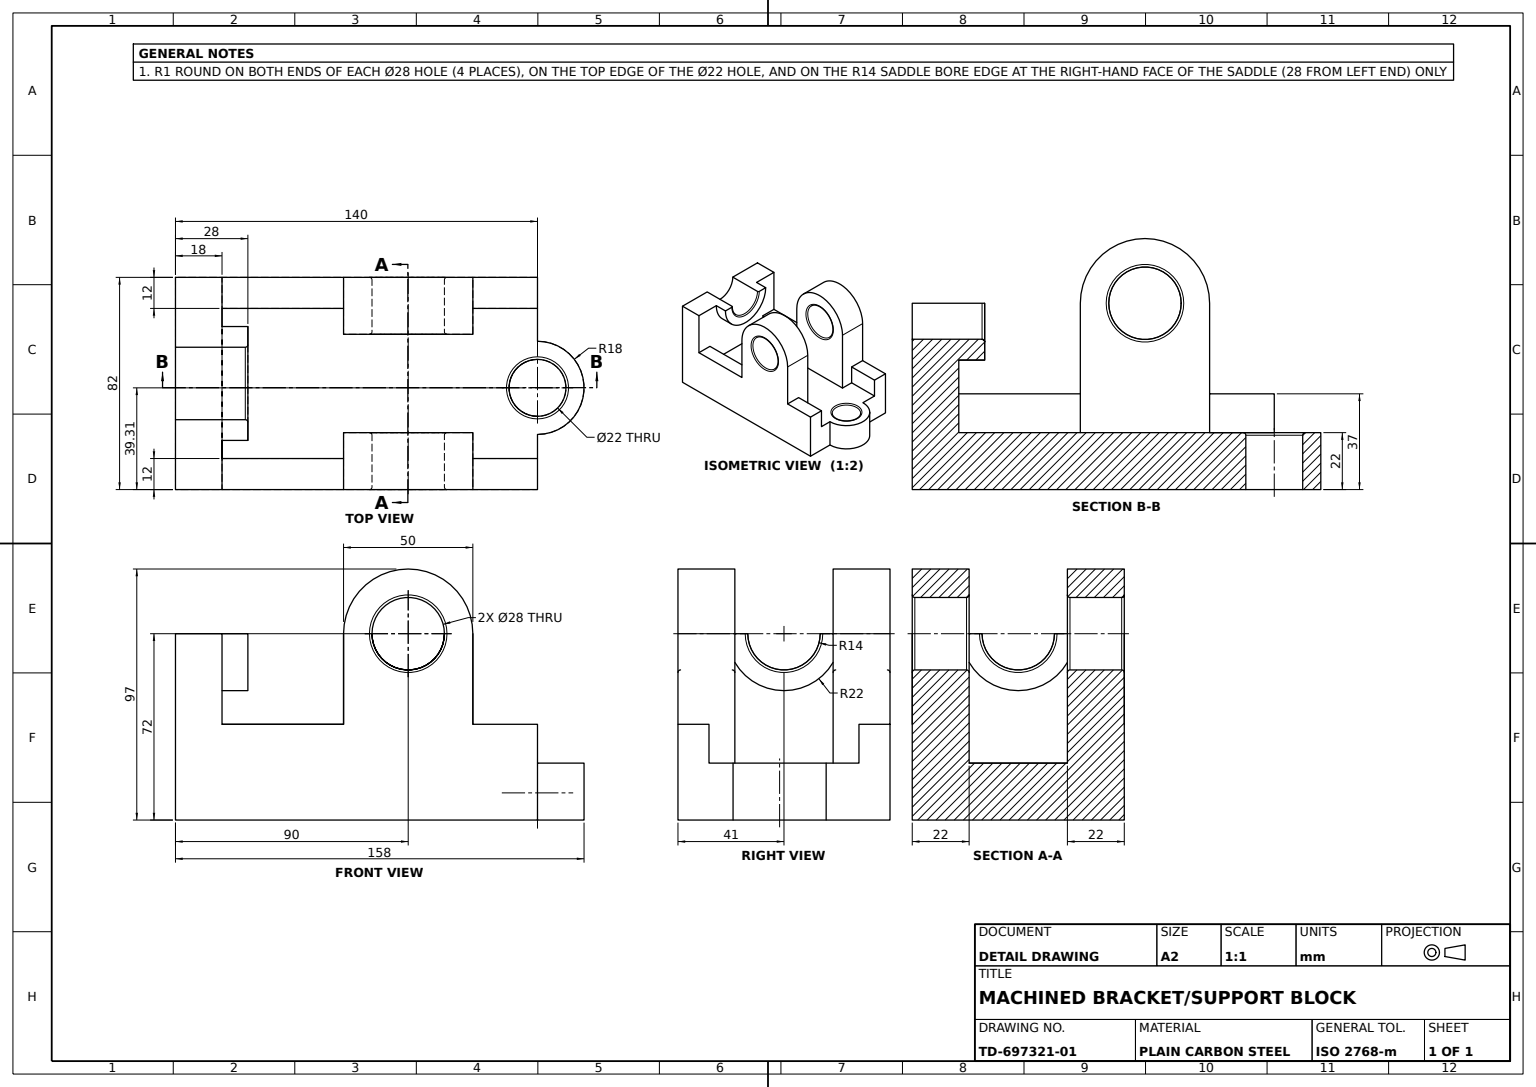
from build123d import *

# Parameters (mm, degrees)
BASE_BLOCK_SKETCH_R     = 11
BASE_BLOCK_DEPTH        = 22
SIDE_WALLS_SKETCH_W     = 25
SIDE_WALLS_SKETCH_H     = 12
SIDE_WALLS_SKETCH_W_2   = 47
SIDE_WALLS_DEPTH        = 15
UPRIGHTS_SKETCH_W       = 50
UPRIGHTS_SKETCH_H       = 22
UPRIGHTS_SKETCH_W_2     = 18
UPRIGHTS_SKETCH_H_2     = 82
UPRIGHTS_DEPTH          = 50
PIVOT_LUGS_SKETCH_R     = 14
PIVOT_LUGS_DEPTH        = 22
LUG_BORE_SKETCH_R       = 14
LUG_BORE_THROUGH_DEPTH  = 82
LUG_START               = -22
LUG_INFILL_DEPTH        = 22
SADDLE_BLOCK_DEPTH      = 28
BASE_EDGE_FILLET_R1_R   = 1
LUG_EDGE_FILLETS_R1_R   = 1
SADDLE_START            = -22
SADDLE_CRADLE_CUT_DEPTH = 22


with BuildPart() as part:
    # Base Block Sketch → Base Block (new body)
    with BuildSketch(Plane(origin=(0, 0, 0), x_dir=(1, 0, 0), z_dir=(0, 1, 0))):
        with BuildLine():
            Line((70, 16.3081571), (70, 41))
            Line((70, 41), (-70, 41))
            Line((-70, 41), (-70, -41))
            Line((-70, -41), (70, -41))
            Line((70, -41), (70, -19.6918429))
            ThreePointArc((70, -19.6918429), (88, -1.6918429), (70, 16.3081571))
        make_face()
        with Locations(Location((70, -1.6918429, 0), (0, 0, 270))):
            Circle(BASE_BLOCK_SKETCH_R, mode=Mode.SUBTRACT)
    extrude(amount=BASE_BLOCK_DEPTH)

    # Side Walls Sketch → Side Walls (add)
    with BuildSketch(Plane(origin=(0, 22, 0), x_dir=(1, 0, 0), z_dir=(0, 1, 0))):
        with Locations((57.5, 35)):
            Rectangle(SIDE_WALLS_SKETCH_W, SIDE_WALLS_SKETCH_H)
        with Locations((-28.5, 35)):
            Rectangle(SIDE_WALLS_SKETCH_W_2, SIDE_WALLS_SKETCH_H)
        with Locations((-28.5, -35)):
            Rectangle(SIDE_WALLS_SKETCH_W_2, SIDE_WALLS_SKETCH_H)
        with Locations((57.5, -35)):
            Rectangle(SIDE_WALLS_SKETCH_W, SIDE_WALLS_SKETCH_H)
    extrude(amount=SIDE_WALLS_DEPTH)

    # Uprights Sketch → Uprights (add)
    with BuildSketch(Plane(origin=(0, 22, 0), x_dir=(1, 0, 0), z_dir=(0, 1, 0))):
        with Locations((20, 30)):
            Rectangle(UPRIGHTS_SKETCH_W, UPRIGHTS_SKETCH_H)
        with Locations((20, -30)):
            Rectangle(UPRIGHTS_SKETCH_W, UPRIGHTS_SKETCH_H)
        with Locations((-61, 0)):
            Rectangle(UPRIGHTS_SKETCH_W_2, UPRIGHTS_SKETCH_H_2)
    extrude(amount=UPRIGHTS_DEPTH)

    # Pivot Lugs Sketch → Pivot Lugs (add)
    with BuildSketch(Plane.XY.offset(41)):
        with BuildLine():
            Line((-5, 72), (-5, 37))
            Line((-5, 37), (45, 37))
            Line((45, 37), (45, 72))
            ThreePointArc((45, 72), (20, 97), (-5, 72))
        make_face()
        with Locations((20, 72)):
            Circle(PIVOT_LUGS_SKETCH_R, mode=Mode.SUBTRACT)
    extrude(amount=-PIVOT_LUGS_DEPTH)

    # Lug Bore Sketch → Lug Bore Through (cut)
    with BuildSketch(Plane.XY.offset(41)):
        with Locations((20, 72)):
            Circle(LUG_BORE_SKETCH_R)
    extrude(amount=-LUG_BORE_THROUGH_DEPTH, mode=Mode.SUBTRACT)

    # Lug Infill Sketch → Lug Infill (add)
    with BuildSketch(Plane(origin=(0, 0, -41), x_dir=(-1, 0, 0), z_dir=(0, 0, -1)).offset(LUG_START)):
        with BuildLine():
            Line((-34, 72), (-45, 72))
            ThreePointArc((-45, 72), (-20, 97), (5, 72))
            Line((5, 72), (-6, 72))
            ThreePointArc((-6, 72), (-20, 86), (-34, 72))
        make_face()
    extrude(amount=LUG_INFILL_DEPTH)

    # Saddle Block Sketch → Saddle Block (add)
    with BuildSketch(Plane.ZY.offset(70)):
        with BuildLine():
            Line((-14, 72), (-22, 72))
            ThreePointArc((-22, 72), (0, 50), (22, 72))
            Line((22, 72), (14, 72))
            ThreePointArc((14, 72), (0, 58), (-14, 72))
        make_face()
    extrude(amount=-SADDLE_BLOCK_DEPTH)

    # Base Edge Fillet R1
    base_edge_fillet_r1_edges = [part.edges().sort_by_distance(p)[0] for p in [
        (70, 22, -9.3081571),
    ]]
    fillet(base_edge_fillet_r1_edges, radius=BASE_EDGE_FILLET_R1_R)

    # Lug Edge Fillets R1
    lug_edge_fillets_r1_edges = [part.edges().sort_by_distance(p)[0] for p in [
        (6, 72, 41),
        (6, 72, 19),
        (34, 72, -41),
        (34, 72, -19),
        (-42, 58, 0),
    ]]
    fillet(lug_edge_fillets_r1_edges, radius=LUG_EDGE_FILLETS_R1_R)

    # Saddle Cradle Sketch → Saddle Cradle Cut (cut)
    with BuildSketch(Plane(origin=(-52, 0, 0), x_dir=(0, 0, -1), z_dir=(1, 0, 0)).offset(SADDLE_START)):
        with BuildLine():
            Line((-14, 72), (14, 72))
            ThreePointArc((14, 72), (0, 58), (-14, 72))
        make_face()
    extrude(amount=SADDLE_CRADLE_CUT_DEPTH, mode=Mode.SUBTRACT)


solid = part.part
